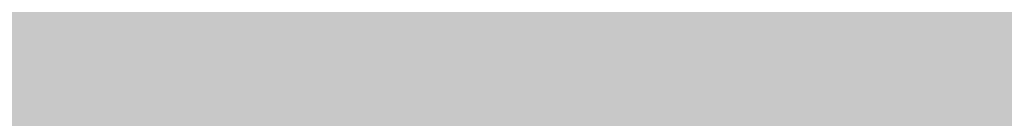
# Model space of a CAD drawing. Units: millimetres. Extents: x -22994 to 29398, y -19990 to 20176.
# Tile 99 of 135: x 229.428 to 230.597, y 84.615 to 84.732. Entities that reach past the tile are written whole.
import ezdxf
from ezdxf import colors
from ezdxf.entities.mleader import LeaderData, LeaderLine
from ezdxf.math import Vec2, Vec3

# ---------------------------------------------------------------- set-up
doc = ezdxf.new("R2010")
doc.units = ezdxf.units.MM
doc.header["$MEASUREMENT"] = 0
doc.layers.add('M-ANNO-TEXT', color=7, linetype='Continuous', lineweight=25)
doc.layers.add('M-DIMS', color=2, linetype='Continuous', lineweight=18)
doc.styles.get("Standard").update_dxf_attribs({"font": 'arial.ttf'})
doc.dimstyles.get("Standard").update_dxf_attribs({"dimtxt": 0.18, "dimasz": 10000, "dimexe": 0.18, "dimexo": 0.0625, "dimgap": 0.09, "dimtad": 0, "dimtih": 1, "dimtoh": 1, "dimdec": 0, "dimzin": 0, "dimdsep": 46, "dimtxsty": 'Standard', "dimcen": 0.09, "dimadec": 0, "dimazin": 0, "dimtfac": 1, "dimtdec": 0, "dimtofl": 0, "dimtmove": 0, "dimatfit": 3, "dimfxl": 1, "dimtolj": 1, "dimtzin": 0, "dimlwd": 30, "dimarcsym": 0})

# ---------------------------------------------------------------- blocks, each defined once
blk = doc.blocks.new('*D2')
at = {"layer": 'Defpoints', "color": 0, "transparency": 16777216}
for p in [(6.6773, 10.2713), (290.852, 10.2713), (290.852, -5.0787)]:
    blk.add_point(p, dxfattribs=at)
at = {"layer": 'M-DIMS', "color": 0, "lineweight": -2, "transparency": 16777216}
for p, q in [((6.6773, 10.2088), (6.6773, -5.2587)), ((290.852, 10.2088), (290.852, -5.2587))]:
    blk.add_line(p, q, dxfattribs=at)
at = {"layer": 'M-DIMS', "color": 0, "lineweight": 30, "transparency": 16777216}
for p, q in [((-9993.3227, -5.0787), (-19993.3227, -5.0787)), ((10290.852, -5.0787), (20290.852, -5.0787))]:
    blk.add_line(p, q, dxfattribs=at)
at = {"layer": 'M-DIMS', "color": 0, "transparency": 16777216}
for points in [[(-9993.3227, 1661.5879), (-9993.3227, -1671.7454), (6.6773, -5.0787)], [(10290.852, 1661.5879), (10290.852, -1671.7454), (290.852, -5.0787)]]:
    blk.add_solid(points, dxfattribs=at)
at = {"layer": 'M-DIMS', "color": 0, "transparency": 16777216, "insert": (148.7647, -5.0787), "char_height": 0.18, "attachment_point": 5}
blk.add_mtext('\\A1;284.2', dxfattribs=at)
blk = doc.blocks.new('*D3')
at = {"layer": 'Defpoints', "color": 0, "transparency": 16777216}
for p in [(110.2647, 204.1654), (110.2647, 176.3662), (95.8327, 127.967)]:
    blk.add_point(p, dxfattribs=at)
at = {"layer": 'M-DIMS', "color": 0, "lineweight": -2, "transparency": 16777216}
for p, q in [((95.8327, 128.0295), (95.8327, 204.3454)), ((110.2647, 176.4287), (110.2647, 204.3454))]:
    blk.add_line(p, q, dxfattribs=at)
at = {"layer": 'M-DIMS', "color": 0, "lineweight": 30, "transparency": 16777216}
for p, q in [((-9904.1673, 204.1654), (-19904.1673, 204.1654)), ((10110.2647, 204.1654), (20110.2647, 204.1654))]:
    blk.add_line(p, q, dxfattribs=at)
at = {"layer": 'M-DIMS', "color": 0, "transparency": 16777216}
for points in [[(-9904.1673, 1870.8321), (-9904.1673, -1462.5013), (95.8327, 204.1654)], [(10110.2647, 1870.8321), (10110.2647, -1462.5013), (110.2647, 204.1654)]]:
    blk.add_solid(points, dxfattribs=at)
at = {"layer": 'M-DIMS', "color": 0, "transparency": 16777216, "insert": (103.0487, 204.1654), "char_height": 0.18, "attachment_point": 5}
blk.add_mtext('\\A1;14.432', dxfattribs=at)
blk = doc.blocks.new('*D4')
at = {"layer": 'Defpoints', "color": 0, "transparency": 16777216}
for p in [(116.2647, 204.1654), (110.2647, 176.3662), (116.2647, 176.3662)]:
    blk.add_point(p, dxfattribs=at)
at = {"layer": 'M-DIMS', "color": 0, "lineweight": -2, "transparency": 16777216}
for p, q in [((110.2647, 176.4287), (110.2647, 204.3454)), ((116.2647, 176.4287), (116.2647, 204.3454))]:
    blk.add_line(p, q, dxfattribs=at)
at = {"layer": 'M-DIMS', "color": 0, "lineweight": 30, "transparency": 16777216}
for p, q in [((-9889.7353, 204.1654), (-19889.7353, 204.1654)), ((10116.2647, 204.1654), (20116.2647, 204.1654))]:
    blk.add_line(p, q, dxfattribs=at)
at = {"layer": 'M-DIMS', "color": 0, "transparency": 16777216}
for points in [[(-9889.7353, 1870.8321), (-9889.7353, -1462.5013), (110.2647, 204.1654)], [(10116.2647, 1870.8321), (10116.2647, -1462.5013), (116.2647, 204.1654)]]:
    blk.add_solid(points, dxfattribs=at)
at = {"layer": 'M-DIMS', "color": 0, "transparency": 16777216, "insert": (113.2647, 204.1654), "char_height": 0.18, "attachment_point": 5}
blk.add_mtext('\\A1;6', dxfattribs=at)
blk = doc.blocks.new('*D5')
at = {"layer": 'Defpoints', "color": 0, "transparency": 16777216}
for p in [(181.2647, 204.1654), (116.2647, 176.3662), (181.2647, 176.3662)]:
    blk.add_point(p, dxfattribs=at)
at = {"layer": 'M-DIMS', "color": 0, "lineweight": -2, "transparency": 16777216}
for p, q in [((116.2647, 176.4287), (116.2647, 204.3454)), ((181.2647, 176.4287), (181.2647, 204.3454))]:
    blk.add_line(p, q, dxfattribs=at)
at = {"layer": 'M-DIMS', "color": 0, "lineweight": 30, "transparency": 16777216}
for p, q in [((-9883.7353, 204.1654), (-19883.7353, 204.1654)), ((10181.2647, 204.1654), (20181.2647, 204.1654))]:
    blk.add_line(p, q, dxfattribs=at)
at = {"layer": 'M-DIMS', "color": 0, "transparency": 16777216}
for points in [[(-9883.7353, 1870.8321), (-9883.7353, -1462.5013), (116.2647, 204.1654)], [(10181.2647, 1870.8321), (10181.2647, -1462.5013), (181.2647, 204.1654)]]:
    blk.add_solid(points, dxfattribs=at)
at = {"layer": 'M-DIMS', "color": 0, "transparency": 16777216, "insert": (148.7647, 204.1654), "char_height": 0.18, "attachment_point": 5}
blk.add_mtext('\\A1;65', dxfattribs=at)
blk = doc.blocks.new('*D6')
at = {"layer": 'Defpoints', "color": 0, "transparency": 16777216}
for p in [(187.2647, 204.1654), (181.2647, 176.3662), (187.2647, 176.3662)]:
    blk.add_point(p, dxfattribs=at)
at = {"layer": 'M-DIMS', "color": 0, "lineweight": -2, "transparency": 16777216}
for p, q in [((181.2647, 176.4287), (181.2647, 204.3454)), ((187.2647, 176.4287), (187.2647, 204.3454))]:
    blk.add_line(p, q, dxfattribs=at)
at = {"layer": 'M-DIMS', "color": 0, "lineweight": 30, "transparency": 16777216}
for p, q in [((-9818.7353, 204.1654), (-19818.7353, 204.1654)), ((10187.2647, 204.1654), (20187.2647, 204.1654))]:
    blk.add_line(p, q, dxfattribs=at)
at = {"layer": 'M-DIMS', "color": 0, "transparency": 16777216}
for points in [[(-9818.7353, 1870.8321), (-9818.7353, -1462.5013), (181.2647, 204.1654)], [(10187.2647, 1870.8321), (10187.2647, -1462.5013), (187.2647, 204.1654)]]:
    blk.add_solid(points, dxfattribs=at)
at = {"layer": 'M-DIMS', "color": 0, "transparency": 16777216, "insert": (184.2647, 204.1654), "char_height": 0.18, "attachment_point": 5}
blk.add_mtext('\\A1;6', dxfattribs=at)
blk = doc.blocks.new('*D7')
at = {"layer": 'Defpoints', "color": 0, "transparency": 16777216}
for p in [(201.6967, 204.1654), (187.2647, 176.3662), (201.6967, 127.967)]:
    blk.add_point(p, dxfattribs=at)
at = {"layer": 'M-DIMS', "color": 0, "lineweight": -2, "transparency": 16777216}
for p, q in [((187.2647, 176.4287), (187.2647, 204.3454)), ((201.6967, 128.0295), (201.6967, 204.3454))]:
    blk.add_line(p, q, dxfattribs=at)
at = {"layer": 'M-DIMS', "color": 0, "lineweight": 30, "transparency": 16777216}
for p, q in [((-9812.7353, 204.1654), (-19812.7353, 204.1654)), ((10201.6967, 204.1654), (20201.6967, 204.1654))]:
    blk.add_line(p, q, dxfattribs=at)
at = {"layer": 'M-DIMS', "color": 0, "transparency": 16777216}
for points in [[(-9812.7353, 1870.8321), (-9812.7353, -1462.5013), (187.2647, 204.1654)], [(10201.6967, 1870.8321), (10201.6967, -1462.5013), (201.6967, 204.1654)]]:
    blk.add_solid(points, dxfattribs=at)
at = {"layer": 'M-DIMS', "color": 0, "transparency": 16777216, "insert": (194.4807, 204.1654), "char_height": 0.18, "attachment_point": 5}
blk.add_mtext('\\A1;14.432', dxfattribs=at)
blk = doc.blocks.new('*D8')
at = {"layer": 'Defpoints', "color": 0, "transparency": 16777216}
for p in [(227.6485, 204.1654), (227.6485, 146.7296), (201.6967, 127.967)]:
    blk.add_point(p, dxfattribs=at)
at = {"layer": 'M-DIMS', "color": 0, "lineweight": -2, "transparency": 16777216}
for p, q in [((201.6967, 128.0295), (201.6967, 204.3454)), ((227.6485, 146.7921), (227.6485, 204.3454))]:
    blk.add_line(p, q, dxfattribs=at)
at = {"layer": 'M-DIMS', "color": 0, "lineweight": 30, "transparency": 16777216}
for p, q in [((-9798.3033, 204.1654), (-19798.3033, 204.1654)), ((10227.6485, 204.1654), (20227.6485, 204.1654))]:
    blk.add_line(p, q, dxfattribs=at)
at = {"layer": 'M-DIMS', "color": 0, "transparency": 16777216}
for points in [[(-9798.3033, 1870.8321), (-9798.3033, -1462.5013), (201.6967, 204.1654)], [(10227.6485, 1870.8321), (10227.6485, -1462.5013), (227.6485, 204.1654)]]:
    blk.add_solid(points, dxfattribs=at)
at = {"layer": 'M-DIMS', "color": 0, "transparency": 16777216, "insert": (214.6726, 204.1654), "char_height": 0.18, "attachment_point": 5}
blk.add_mtext('\\A1;25.95', dxfattribs=at)
blk = doc.blocks.new('*D9')
at = {"layer": 'Defpoints', "color": 0, "transparency": 16777216}
for p in [(187.2647, 176.3662), (306.202, 176.3662), (290.852, 10.2713)]:
    blk.add_point(p, dxfattribs=at)
at = {"layer": 'M-DIMS', "color": 0, "lineweight": 30, "transparency": 16777216}
for p, q in [((306.202, 10176.3662), (306.202, 20176.3662)), ((306.202, -9989.7287), (306.202, -19989.7287))]:
    blk.add_line(p, q, dxfattribs=at)
at = {"layer": 'M-DIMS', "color": 0, "lineweight": -2, "transparency": 16777216}
for p, q in [((187.3272, 176.3662), (306.382, 176.3662)), ((290.9145, 10.2713), (306.382, 10.2713))]:
    blk.add_line(p, q, dxfattribs=at)
at = {"layer": 'M-DIMS', "color": 0, "transparency": 16777216}
for points in [[(-1360.4646, 10176.3662), (1972.8687, 10176.3662), (306.202, 176.3662)], [(-1360.4646, -9989.7287), (1972.8687, -9989.7287), (306.202, 10.2713)]]:
    blk.add_solid(points, dxfattribs=at)
at = {"layer": 'M-DIMS', "color": 0, "transparency": 16777216, "insert": (306.202, 93.3187), "char_height": 0.18, "attachment_point": 5}
blk.add_mtext('\\A1;166.1', dxfattribs=at)
blk = doc.blocks.new('*D10')
at = {"layer": 'Defpoints', "color": 0, "transparency": 16777216}
for p in [(125.6498, 136.0713), (133.3459, 136.0713), (133.3459, -5.0787)]:
    blk.add_point(p, dxfattribs=at)
at = {"layer": 'M-DIMS', "color": 0, "lineweight": -2, "transparency": 16777216}
for p, q in [((125.6498, 136.0088), (125.6498, -5.2587)), ((133.3459, 136.0088), (133.3459, -5.2587))]:
    blk.add_line(p, q, dxfattribs=at)
at = {"layer": 'M-DIMS', "color": 0, "lineweight": 30, "transparency": 16777216}
for p, q in [((-9874.3502, -5.0787), (-19874.3502, -5.0787)), ((10133.3459, -5.0787), (20133.3459, -5.0787))]:
    blk.add_line(p, q, dxfattribs=at)
at = {"layer": 'M-DIMS', "color": 0, "transparency": 16777216}
for points in [[(-9874.3502, 1661.5879), (-9874.3502, -1671.7454), (125.6498, -5.0787)], [(10133.3459, 1661.5879), (10133.3459, -1671.7454), (133.3459, -5.0787)]]:
    blk.add_solid(points, dxfattribs=at)
at = {"layer": 'M-DIMS', "color": 0, "transparency": 16777216, "insert": (129.4978, -5.0787), "char_height": 0.18, "attachment_point": 5}
blk.add_mtext('\\A1;7.696', dxfattribs=at)
blk = doc.blocks.new('*D11')
at = {"layer": 'Defpoints', "color": 0, "transparency": 16777216}
for p in [(133.3459, 136.0713), (135.6498, 136.0713), (135.6498, -5.0787)]:
    blk.add_point(p, dxfattribs=at)
at = {"layer": 'M-DIMS', "color": 0, "lineweight": -2, "transparency": 16777216}
for p, q in [((133.3459, 136.0088), (133.3459, -5.2587)), ((135.6498, 136.0088), (135.6498, -5.2587))]:
    blk.add_line(p, q, dxfattribs=at)
at = {"layer": 'M-DIMS', "color": 0, "lineweight": 30, "transparency": 16777216}
for p, q in [((-9866.6541, -5.0787), (-19866.6541, -5.0787)), ((10135.6498, -5.0787), (20135.6498, -5.0787))]:
    blk.add_line(p, q, dxfattribs=at)
at = {"layer": 'M-DIMS', "color": 0, "transparency": 16777216}
for points in [[(-9866.6541, 1661.5879), (-9866.6541, -1671.7454), (133.3459, -5.0787)], [(10135.6498, 1661.5879), (10135.6498, -1671.7454), (135.6498, -5.0787)]]:
    blk.add_solid(points, dxfattribs=at)
at = {"layer": 'M-DIMS', "color": 0, "transparency": 16777216, "insert": (134.4978, -5.0787), "char_height": 0.18, "attachment_point": 5}
blk.add_mtext('\\A1;2.304', dxfattribs=at)
blk = doc.blocks.new('*D12')
at = {"layer": 'Defpoints', "color": 0, "transparency": 16777216}
for p in [(135.6498, 136.0713), (145.6498, 136.0713), (145.6498, -5.0787)]:
    blk.add_point(p, dxfattribs=at)
at = {"layer": 'M-DIMS', "color": 0, "lineweight": -2, "transparency": 16777216}
for p, q in [((135.6498, 136.0088), (135.6498, -5.2587)), ((145.6498, 136.0088), (145.6498, -5.2587))]:
    blk.add_line(p, q, dxfattribs=at)
at = {"layer": 'M-DIMS', "color": 0, "lineweight": 30, "transparency": 16777216}
for p, q in [((-9864.3502, -5.0787), (-19864.3502, -5.0787)), ((10145.6498, -5.0787), (20145.6498, -5.0787))]:
    blk.add_line(p, q, dxfattribs=at)
at = {"layer": 'M-DIMS', "color": 0, "transparency": 16777216}
for points in [[(-9864.3502, 1661.5879), (-9864.3502, -1671.7454), (135.6498, -5.0787)], [(10145.6498, 1661.5879), (10145.6498, -1671.7454), (145.6498, -5.0787)]]:
    blk.add_solid(points, dxfattribs=at)
at = {"layer": 'M-DIMS', "color": 0, "transparency": 16777216, "insert": (140.6498, -5.0787), "char_height": 0.18, "attachment_point": 5}
blk.add_mtext('\\A1;10', dxfattribs=at)
blk = doc.blocks.new('*D13')
at = {"layer": 'Defpoints', "color": 0, "transparency": 16777216}
for p in [(145.6498, 136.0713), (155.6498, 136.0713), (155.6498, -5.0787)]:
    blk.add_point(p, dxfattribs=at)
at = {"layer": 'M-DIMS', "color": 0, "lineweight": -2, "transparency": 16777216}
for p, q in [((145.6498, 136.0088), (145.6498, -5.2587)), ((155.6498, 136.0088), (155.6498, -5.2587))]:
    blk.add_line(p, q, dxfattribs=at)
at = {"layer": 'M-DIMS', "color": 0, "lineweight": 30, "transparency": 16777216}
for p, q in [((-9854.3502, -5.0787), (-19854.3502, -5.0787)), ((10155.6498, -5.0787), (20155.6498, -5.0787))]:
    blk.add_line(p, q, dxfattribs=at)
at = {"layer": 'M-DIMS', "color": 0, "transparency": 16777216}
for points in [[(-9854.3502, 1661.5879), (-9854.3502, -1671.7454), (145.6498, -5.0787)], [(10155.6498, 1661.5879), (10155.6498, -1671.7454), (155.6498, -5.0787)]]:
    blk.add_solid(points, dxfattribs=at)
at = {"layer": 'M-DIMS', "color": 0, "transparency": 16777216, "insert": (150.6498, -5.0787), "char_height": 0.18, "attachment_point": 5}
blk.add_mtext('\\A1;10', dxfattribs=at)
blk = doc.blocks.new('*D14')
at = {"layer": 'Defpoints', "color": 0, "transparency": 16777216}
for p in [(155.6498, 136.0713), (165.6498, 136.0713), (165.6498, -5.0787)]:
    blk.add_point(p, dxfattribs=at)
at = {"layer": 'M-DIMS', "color": 0, "lineweight": -2, "transparency": 16777216}
for p, q in [((155.6498, 136.0088), (155.6498, -5.2587)), ((165.6498, 136.0088), (165.6498, -5.2587))]:
    blk.add_line(p, q, dxfattribs=at)
at = {"layer": 'M-DIMS', "color": 0, "lineweight": 30, "transparency": 16777216}
for p, q in [((-9844.3502, -5.0787), (-19844.3502, -5.0787)), ((10165.6498, -5.0787), (20165.6498, -5.0787))]:
    blk.add_line(p, q, dxfattribs=at)
at = {"layer": 'M-DIMS', "color": 0, "transparency": 16777216}
for points in [[(-9844.3502, 1661.5879), (-9844.3502, -1671.7454), (155.6498, -5.0787)], [(10165.6498, 1661.5879), (10165.6498, -1671.7454), (165.6498, -5.0787)]]:
    blk.add_solid(points, dxfattribs=at)
at = {"layer": 'M-DIMS', "color": 0, "transparency": 16777216, "insert": (160.6498, -5.0787), "char_height": 0.18, "attachment_point": 5}
blk.add_mtext('\\A1;10', dxfattribs=at)
blk = doc.blocks.new('*D15')
at = {"layer": 'Defpoints', "color": 0, "transparency": 16777216}
for p in [(173.3459, 154.788), (173.3459, 136.0713), (306.202, 136.0713)]:
    blk.add_point(p, dxfattribs=at)
at = {"layer": 'M-DIMS', "color": 0, "lineweight": 30, "transparency": 16777216}
for p, q in [((306.202, 10154.788), (306.202, 20154.788)), ((306.202, -9863.9287), (306.202, -19863.9287))]:
    blk.add_line(p, q, dxfattribs=at)
at = {"layer": 'M-DIMS', "color": 0, "lineweight": -2, "transparency": 16777216}
for p, q in [((173.4084, 154.788), (306.382, 154.788)), ((173.4084, 136.0713), (306.382, 136.0713))]:
    blk.add_line(p, q, dxfattribs=at)
at = {"layer": 'M-DIMS', "color": 0, "transparency": 16777216}
for points in [[(-1360.4646, 10154.788), (1972.8687, 10154.788), (306.202, 154.788)], [(-1360.4646, -9863.9287), (1972.8687, -9863.9287), (306.202, 136.0713)]]:
    blk.add_solid(points, dxfattribs=at)
at = {"layer": 'M-DIMS', "color": 0, "transparency": 16777216, "insert": (306.202, 145.4297), "char_height": 0.18, "attachment_point": 5}
blk.add_mtext('\\A1;18.717', dxfattribs=at)
blk = doc.blocks.new('*D16')
at = {"layer": 'Defpoints', "color": 0, "transparency": 16777216}
for p in [(120.1702, 204.1654), (110.4658, 48.0349), (120.1702, 48.0349)]:
    blk.add_point(p, dxfattribs=at)
at = {"layer": 'M-DIMS', "color": 0, "lineweight": -2, "transparency": 16777216}
for p, q in [((110.4658, 48.0974), (110.4658, 204.3454)), ((120.1702, 48.0974), (120.1702, 204.3454))]:
    blk.add_line(p, q, dxfattribs=at)
at = {"layer": 'M-DIMS', "color": 0, "lineweight": 30, "transparency": 16777216}
for p, q in [((-9889.5342, 204.1654), (-19889.5342, 204.1654)), ((10120.1702, 204.1654), (20120.1702, 204.1654))]:
    blk.add_line(p, q, dxfattribs=at)
at = {"layer": 'M-DIMS', "color": 0, "transparency": 16777216}
for points in [[(-9889.5342, 1870.8321), (-9889.5342, -1462.5013), (110.4658, 204.1654)], [(10120.1702, 1870.8321), (10120.1702, -1462.5013), (120.1702, 204.1654)]]:
    blk.add_solid(points, dxfattribs=at)
at = {"layer": 'M-DIMS', "color": 0, "transparency": 16777216, "insert": (115.318, 204.1654), "char_height": 0.18, "attachment_point": 5}
blk.add_mtext('\\A1;9.704', dxfattribs=at)
blk = doc.blocks.new('*D17')
at = {"layer": 'Defpoints', "color": 0, "transparency": 16777216}
for p in [(126.1702, 204.1654), (120.1702, 48.0349), (126.1702, 48.0349)]:
    blk.add_point(p, dxfattribs=at)
at = {"layer": 'M-DIMS', "color": 0, "lineweight": -2, "transparency": 16777216}
for p, q in [((120.1702, 48.0974), (120.1702, 204.3454)), ((126.1702, 48.0974), (126.1702, 204.3454))]:
    blk.add_line(p, q, dxfattribs=at)
at = {"layer": 'M-DIMS', "color": 0, "lineweight": 30, "transparency": 16777216}
for p, q in [((-9879.8298, 204.1654), (-19879.8298, 204.1654)), ((10126.1702, 204.1654), (20126.1702, 204.1654))]:
    blk.add_line(p, q, dxfattribs=at)
at = {"layer": 'M-DIMS', "color": 0, "transparency": 16777216}
for points in [[(-9879.8298, 1870.8321), (-9879.8298, -1462.5013), (120.1702, 204.1654)], [(10126.1702, 1870.8321), (10126.1702, -1462.5013), (126.1702, 204.1654)]]:
    blk.add_solid(points, dxfattribs=at)
at = {"layer": 'M-DIMS', "color": 0, "transparency": 16777216, "insert": (123.1702, 204.1654), "char_height": 0.18, "attachment_point": 5}
blk.add_mtext('\\A1;6', dxfattribs=at)
blk = doc.blocks.new('*D18')
at = {"layer": 'Defpoints', "color": 0, "transparency": 16777216}
for p in [(132.1702, 204.1654), (126.1702, 48.0349), (132.1702, 48.0349)]:
    blk.add_point(p, dxfattribs=at)
at = {"layer": 'M-DIMS', "color": 0, "lineweight": -2, "transparency": 16777216}
for p, q in [((126.1702, 48.0974), (126.1702, 204.3454)), ((132.1702, 48.0974), (132.1702, 204.3454))]:
    blk.add_line(p, q, dxfattribs=at)
at = {"layer": 'M-DIMS', "color": 0, "lineweight": 30, "transparency": 16777216}
for p, q in [((-9873.8298, 204.1654), (-19873.8298, 204.1654)), ((10132.1702, 204.1654), (20132.1702, 204.1654))]:
    blk.add_line(p, q, dxfattribs=at)
at = {"layer": 'M-DIMS', "color": 0, "transparency": 16777216}
for points in [[(-9873.8298, 1870.8321), (-9873.8298, -1462.5013), (126.1702, 204.1654)], [(10132.1702, 1870.8321), (10132.1702, -1462.5013), (132.1702, 204.1654)]]:
    blk.add_solid(points, dxfattribs=at)
at = {"layer": 'M-DIMS', "color": 0, "transparency": 16777216, "insert": (129.1702, 204.1654), "char_height": 0.18, "attachment_point": 5}
blk.add_mtext('\\A1;6', dxfattribs=at)
blk = doc.blocks.new('*D19')
at = {"layer": 'Defpoints', "color": 0, "transparency": 16777216}
for p in [(138.1702, 204.1654), (132.1702, 48.0349), (138.1702, 48.0349)]:
    blk.add_point(p, dxfattribs=at)
at = {"layer": 'M-DIMS', "color": 0, "lineweight": -2, "transparency": 16777216}
for p, q in [((132.1702, 48.0974), (132.1702, 204.3454)), ((138.1702, 48.0974), (138.1702, 204.3454))]:
    blk.add_line(p, q, dxfattribs=at)
at = {"layer": 'M-DIMS', "color": 0, "lineweight": 30, "transparency": 16777216}
for p, q in [((-9867.8298, 204.1654), (-19867.8298, 204.1654)), ((10138.1702, 204.1654), (20138.1702, 204.1654))]:
    blk.add_line(p, q, dxfattribs=at)
at = {"layer": 'M-DIMS', "color": 0, "transparency": 16777216}
for points in [[(-9867.8298, 1870.8321), (-9867.8298, -1462.5013), (132.1702, 204.1654)], [(10138.1702, 1870.8321), (10138.1702, -1462.5013), (138.1702, 204.1654)]]:
    blk.add_solid(points, dxfattribs=at)
at = {"layer": 'M-DIMS', "color": 0, "transparency": 16777216, "insert": (135.1702, 204.1654), "char_height": 0.18, "attachment_point": 5}
blk.add_mtext('\\A1;6', dxfattribs=at)
blk = doc.blocks.new('*D20')
at = {"layer": 'Defpoints', "color": 0, "transparency": 16777216}
for p in [(144.1702, 204.1654), (138.1702, 48.0349), (144.1702, 48.0349)]:
    blk.add_point(p, dxfattribs=at)
at = {"layer": 'M-DIMS', "color": 0, "lineweight": -2, "transparency": 16777216}
for p, q in [((138.1702, 48.0974), (138.1702, 204.3454)), ((144.1702, 48.0974), (144.1702, 204.3454))]:
    blk.add_line(p, q, dxfattribs=at)
at = {"layer": 'M-DIMS', "color": 0, "lineweight": 30, "transparency": 16777216}
for p, q in [((-9861.8298, 204.1654), (-19861.8298, 204.1654)), ((10144.1702, 204.1654), (20144.1702, 204.1654))]:
    blk.add_line(p, q, dxfattribs=at)
at = {"layer": 'M-DIMS', "color": 0, "transparency": 16777216}
for points in [[(-9861.8298, 1870.8321), (-9861.8298, -1462.5013), (138.1702, 204.1654)], [(10144.1702, 1870.8321), (10144.1702, -1462.5013), (144.1702, 204.1654)]]:
    blk.add_solid(points, dxfattribs=at)
at = {"layer": 'M-DIMS', "color": 0, "transparency": 16777216, "insert": (141.1702, 204.1654), "char_height": 0.18, "attachment_point": 5}
blk.add_mtext('\\A1;6', dxfattribs=at)
blk = doc.blocks.new('*D21')
at = {"layer": 'Defpoints', "color": 0, "transparency": 16777216}
for p in [(149.1157, 204.1654), (144.1702, 48.0349), (149.1157, 48.0349)]:
    blk.add_point(p, dxfattribs=at)
at = {"layer": 'M-DIMS', "color": 0, "lineweight": -2, "transparency": 16777216}
for p, q in [((144.1702, 48.0974), (144.1702, 204.3454)), ((149.1157, 48.0974), (149.1157, 204.3454))]:
    blk.add_line(p, q, dxfattribs=at)
at = {"layer": 'M-DIMS', "color": 0, "lineweight": 30, "transparency": 16777216}
for p, q in [((-9855.8298, 204.1654), (-19855.8298, 204.1654)), ((10149.1157, 204.1654), (20149.1157, 204.1654))]:
    blk.add_line(p, q, dxfattribs=at)
at = {"layer": 'M-DIMS', "color": 0, "transparency": 16777216}
for points in [[(-9855.8298, 1870.8321), (-9855.8298, -1462.5013), (144.1702, 204.1654)], [(10149.1157, 1870.8321), (10149.1157, -1462.5013), (149.1157, 204.1654)]]:
    blk.add_solid(points, dxfattribs=at)
at = {"layer": 'M-DIMS', "color": 0, "transparency": 16777216, "insert": (146.6429, 204.1654), "char_height": 0.18, "attachment_point": 5}
blk.add_mtext('\\A1;4.945', dxfattribs=at)
blk = doc.blocks.new('*D22')
at = {"layer": 'Defpoints', "color": 0, "transparency": 16777216}
for p in [(149.1157, 30.9895), (155.1157, 30.9895), (155.1157, -5.0787)]:
    blk.add_point(p, dxfattribs=at)
at = {"layer": 'M-DIMS', "color": 0, "lineweight": -2, "transparency": 16777216}
for p, q in [((149.1157, 30.927), (149.1157, -5.2587)), ((155.1157, 30.927), (155.1157, -5.2587))]:
    blk.add_line(p, q, dxfattribs=at)
at = {"layer": 'M-DIMS', "color": 0, "lineweight": 30, "transparency": 16777216}
for p, q in [((-9850.8843, -5.0787), (-19850.8843, -5.0787)), ((10155.1157, -5.0787), (20155.1157, -5.0787))]:
    blk.add_line(p, q, dxfattribs=at)
at = {"layer": 'M-DIMS', "color": 0, "transparency": 16777216}
for points in [[(-9850.8843, 1661.5879), (-9850.8843, -1671.7454), (149.1157, -5.0787)], [(10155.1157, 1661.5879), (10155.1157, -1671.7454), (155.1157, -5.0787)]]:
    blk.add_solid(points, dxfattribs=at)
at = {"layer": 'M-DIMS', "color": 0, "transparency": 16777216, "insert": (152.1157, -5.0787), "char_height": 0.18, "attachment_point": 5}
blk.add_mtext('\\A1;6', dxfattribs=at)
blk = doc.blocks.new('*D23')
at = {"layer": 'Defpoints', "color": 0, "transparency": 16777216}
for p in [(155.1157, 30.9895), (161.1157, 30.9895), (161.1157, -5.0787)]:
    blk.add_point(p, dxfattribs=at)
at = {"layer": 'M-DIMS', "color": 0, "lineweight": -2, "transparency": 16777216}
for p, q in [((155.1157, 30.927), (155.1157, -5.2587)), ((161.1157, 30.927), (161.1157, -5.2587))]:
    blk.add_line(p, q, dxfattribs=at)
at = {"layer": 'M-DIMS', "color": 0, "lineweight": 30, "transparency": 16777216}
for p, q in [((-9844.8843, -5.0787), (-19844.8843, -5.0787)), ((10161.1157, -5.0787), (20161.1157, -5.0787))]:
    blk.add_line(p, q, dxfattribs=at)
at = {"layer": 'M-DIMS', "color": 0, "transparency": 16777216}
for points in [[(-9844.8843, 1661.5879), (-9844.8843, -1671.7454), (155.1157, -5.0787)], [(10161.1157, 1661.5879), (10161.1157, -1671.7454), (161.1157, -5.0787)]]:
    blk.add_solid(points, dxfattribs=at)
at = {"layer": 'M-DIMS', "color": 0, "transparency": 16777216, "insert": (158.1157, -5.0787), "char_height": 0.18, "attachment_point": 5}
blk.add_mtext('\\A1;6', dxfattribs=at)
blk = doc.blocks.new('*D24')
at = {"layer": 'Defpoints', "color": 0, "transparency": 16777216}
for p in [(161.1157, 30.9895), (166.4387, 30.9895), (166.4387, -5.0787)]:
    blk.add_point(p, dxfattribs=at)
at = {"layer": 'M-DIMS', "color": 0, "lineweight": -2, "transparency": 16777216}
for p, q in [((161.1157, 30.927), (161.1157, -5.2587)), ((166.4387, 30.927), (166.4387, -5.2587))]:
    blk.add_line(p, q, dxfattribs=at)
at = {"layer": 'M-DIMS', "color": 0, "lineweight": 30, "transparency": 16777216}
for p, q in [((-9838.8843, -5.0787), (-19838.8843, -5.0787)), ((10166.4387, -5.0787), (20166.4387, -5.0787))]:
    blk.add_line(p, q, dxfattribs=at)
at = {"layer": 'M-DIMS', "color": 0, "transparency": 16777216}
for points in [[(-9838.8843, 1661.5879), (-9838.8843, -1671.7454), (161.1157, -5.0787)], [(10166.4387, 1661.5879), (10166.4387, -1671.7454), (166.4387, -5.0787)]]:
    blk.add_solid(points, dxfattribs=at)
at = {"layer": 'M-DIMS', "color": 0, "transparency": 16777216, "insert": (163.7772, -5.0787), "char_height": 0.18, "attachment_point": 5}
blk.add_mtext('\\A1;5.323', dxfattribs=at)
blk = doc.blocks.new('*D25')
at = {"layer": 'Defpoints', "color": 0, "transparency": 16777216}
for p in [(166.4387, 30.9895), (172.4387, 30.9895), (172.4387, -5.0787)]:
    blk.add_point(p, dxfattribs=at)
at = {"layer": 'M-DIMS', "color": 0, "lineweight": -2, "transparency": 16777216}
for p, q in [((166.4387, 30.927), (166.4387, -5.2587)), ((172.4387, 30.927), (172.4387, -5.2587))]:
    blk.add_line(p, q, dxfattribs=at)
at = {"layer": 'M-DIMS', "color": 0, "lineweight": 30, "transparency": 16777216}
for p, q in [((-9833.5613, -5.0787), (-19833.5613, -5.0787)), ((10172.4387, -5.0787), (20172.4387, -5.0787))]:
    blk.add_line(p, q, dxfattribs=at)
at = {"layer": 'M-DIMS', "color": 0, "transparency": 16777216}
for points in [[(-9833.5613, 1661.5879), (-9833.5613, -1671.7454), (166.4387, -5.0787)], [(10172.4387, 1661.5879), (10172.4387, -1671.7454), (172.4387, -5.0787)]]:
    blk.add_solid(points, dxfattribs=at)
at = {"layer": 'M-DIMS', "color": 0, "transparency": 16777216, "insert": (169.4387, -5.0787), "char_height": 0.18, "attachment_point": 5}
blk.add_mtext('\\A1;6', dxfattribs=at)
blk = doc.blocks.new('*D26')
at = {"layer": 'Defpoints', "color": 0, "transparency": 16777216}
for p in [(172.4387, 30.9895), (178.4387, 30.9895), (178.4387, -5.0787)]:
    blk.add_point(p, dxfattribs=at)
at = {"layer": 'M-DIMS', "color": 0, "lineweight": -2, "transparency": 16777216}
for p, q in [((172.4387, 30.927), (172.4387, -5.2587)), ((178.4387, 30.927), (178.4387, -5.2587))]:
    blk.add_line(p, q, dxfattribs=at)
at = {"layer": 'M-DIMS', "color": 0, "lineweight": 30, "transparency": 16777216}
for p, q in [((-9827.5613, -5.0787), (-19827.5613, -5.0787)), ((10178.4387, -5.0787), (20178.4387, -5.0787))]:
    blk.add_line(p, q, dxfattribs=at)
at = {"layer": 'M-DIMS', "color": 0, "transparency": 16777216}
for points in [[(-9827.5613, 1661.5879), (-9827.5613, -1671.7454), (172.4387, -5.0787)], [(10178.4387, 1661.5879), (10178.4387, -1671.7454), (178.4387, -5.0787)]]:
    blk.add_solid(points, dxfattribs=at)
at = {"layer": 'M-DIMS', "color": 0, "transparency": 16777216, "insert": (175.4387, -5.0787), "char_height": 0.18, "attachment_point": 5}
blk.add_mtext('\\A1;6', dxfattribs=at)
blk = doc.blocks.new('*D27')
at = {"layer": 'Defpoints', "color": 0, "transparency": 16777216}
for p in [(178.4387, 30.9895), (188.1175, 30.9895), (188.1175, -5.0787)]:
    blk.add_point(p, dxfattribs=at)
at = {"layer": 'M-DIMS', "color": 0, "lineweight": -2, "transparency": 16777216}
for p, q in [((178.4387, 30.927), (178.4387, -5.2587)), ((188.1175, 30.927), (188.1175, -5.2587))]:
    blk.add_line(p, q, dxfattribs=at)
at = {"layer": 'M-DIMS', "color": 0, "lineweight": 30, "transparency": 16777216}
for p, q in [((-9821.5613, -5.0787), (-19821.5613, -5.0787)), ((10188.1175, -5.0787), (20188.1175, -5.0787))]:
    blk.add_line(p, q, dxfattribs=at)
at = {"layer": 'M-DIMS', "color": 0, "transparency": 16777216}
for points in [[(-9821.5613, 1661.5879), (-9821.5613, -1671.7454), (178.4387, -5.0787)], [(10188.1175, 1661.5879), (10188.1175, -1671.7454), (188.1175, -5.0787)]]:
    blk.add_solid(points, dxfattribs=at)
at = {"layer": 'M-DIMS', "color": 0, "transparency": 16777216, "insert": (183.2781, -5.0787), "char_height": 0.18, "attachment_point": 5}
blk.add_mtext('\\A1;9.679', dxfattribs=at)
blk = doc.blocks.new('*D28')
at = {"layer": 'Defpoints', "color": 0, "transparency": 16777216}
for p in [(188.1175, 48.0349), (306.202, 48.0349), (188.1175, 30.9895)]:
    blk.add_point(p, dxfattribs=at)
at = {"layer": 'M-DIMS', "color": 0, "lineweight": 30, "transparency": 16777216}
for p, q in [((306.202, 10048.0349), (306.202, 20048.0349)), ((306.202, -9969.0105), (306.202, -19969.0105))]:
    blk.add_line(p, q, dxfattribs=at)
at = {"layer": 'M-DIMS', "color": 0, "lineweight": -2, "transparency": 16777216}
for p, q in [((188.18, 48.0349), (306.382, 48.0349)), ((188.18, 30.9895), (306.382, 30.9895))]:
    blk.add_line(p, q, dxfattribs=at)
at = {"layer": 'M-DIMS', "color": 0, "transparency": 16777216}
for points in [[(-1360.4646, 10048.0349), (1972.8687, 10048.0349), (306.202, 48.0349)], [(-1360.4646, -9969.0105), (1972.8687, -9969.0105), (306.202, 30.9895)]]:
    blk.add_solid(points, dxfattribs=at)
at = {"layer": 'M-DIMS', "color": 0, "transparency": 16777216, "insert": (306.202, 39.5122), "char_height": 0.18, "attachment_point": 5}
blk.add_mtext('\\A1;17.045', dxfattribs=at)
blk = doc.blocks.new('*D29')
at = {"layer": 'Defpoints', "color": 0, "transparency": 16777216}
for p in [(36.8006, 80.045), (64.0296, 80.045)]:
    blk.add_point(p, dxfattribs=at)
at = {"layer": 'M-DIMS', "color": 0, "lineweight": -2, "transparency": 16777216}
for p, q in [((50.4151, 79.955), (50.4151, 80.135)), ((50.3251, 80.045), (50.5051, 80.045))]:
    blk.add_line(p, q, dxfattribs=at)
at = {"layer": 'M-DIMS', "color": 0, "lineweight": 30, "transparency": 16777216}
blk.add_line((20064.0296, 80.0303), (10064.0296, 80.0377), dxfattribs=at)
at = {"layer": 'M-DIMS', "color": 0, "transparency": 16777216}
blk.add_solid([(10064.0309, 1746.7043), (10064.0284, -1586.629), (64.0296, 80.045)], dxfattribs=at)
at = {"layer": 'M-DIMS', "color": 0, "transparency": 16777216, "insert": (20064.5213, 80.0303), "char_height": 0.18, "attachment_point": 5}
blk.add_mtext('\\A1;∅27.23', dxfattribs=at)
blk = doc.blocks.new('*D30')
at = {"layer": 'Defpoints', "color": 0, "transparency": 16777216}
for p in [(216.3148, 146.7291), (238.9821, 146.73)]:
    blk.add_point(p, dxfattribs=at)
at = {"layer": 'M-DIMS', "color": 0, "lineweight": 30, "transparency": 16777216}
blk.add_line((20238.9821, 147.4959), (10238.9821, 147.1129), dxfattribs=at)
at = {"layer": 'M-DIMS', "color": 0, "lineweight": -2, "transparency": 16777216}
for p, q in [((227.6485, 146.6396), (227.6485, 146.8196)), ((227.5585, 146.7296), (227.7385, 146.7296))]:
    blk.add_line(p, q, dxfattribs=at)
at = {"layer": 'M-DIMS', "color": 0, "transparency": 16777216}
blk.add_solid([(10238.9183, 1813.7796), (10239.0459, -1519.5537), (238.9821, 146.73)], dxfattribs=at)
at = {"layer": 'M-DIMS', "color": 0, "transparency": 16777216, "insert": (20239.5436, 147.4959), "char_height": 0.18, "attachment_point": 5}
blk.add_mtext('\\A1;∅22.667', dxfattribs=at)
blk = doc.blocks.new('*D31')
at = {"layer": 'Defpoints', "color": 0, "transparency": 16777216}
for p in [(223.1641, 146.7291), (232.1328, 146.73)]:
    blk.add_point(p, dxfattribs=at)
at = {"layer": 'M-DIMS', "color": 0, "lineweight": 30, "transparency": 16777216}
blk.add_line((20232.1327, 148.6656), (10232.1328, 147.6978), dxfattribs=at)
at = {"layer": 'M-DIMS', "color": 0, "lineweight": -2, "transparency": 16777216}
for p, q in [((227.6485, 146.6396), (227.6485, 146.8196)), ((227.5585, 146.7296), (227.7385, 146.7296))]:
    blk.add_line(p, q, dxfattribs=at)
at = {"layer": 'M-DIMS', "color": 0, "transparency": 16777216}
blk.add_solid([(10231.9715, 1814.3645), (10232.2941, -1518.9688), (232.1328, 146.73)], dxfattribs=at)
at = {"layer": 'M-DIMS', "color": 0, "transparency": 16777216, "insert": (20232.6245, 148.6656), "char_height": 0.18, "attachment_point": 5}
blk.add_mtext('\\A1;∅8.969', dxfattribs=at)
blk = doc.blocks.new('*D33')
at = {"layer": 'Defpoints', "color": 0, "transparency": 16777216}
for p in [(229.5613, 154.3773), (232.9972, 153.3509)]:
    blk.add_point(p, dxfattribs=at)
at = {"layer": 'M-DIMS', "color": 0, "lineweight": -2, "transparency": 16777216}
for p, q in [((229.5613, 154.2873), (229.5613, 154.4673)), ((229.4713, 154.3773), (229.6513, 154.3773))]:
    blk.add_line(p, q, dxfattribs=at)
at = {"layer": 'M-DIMS', "color": 0, "lineweight": 30, "transparency": 16777216}
for p, q in [((19396.3388, -5570.8378), (9814.668, -2708.7434)), ((29396.3388, -5570.8378), (19396.3388, -5570.8378))]:
    blk.add_line(p, q, dxfattribs=at)
at = {"layer": 'M-DIMS', "color": 0, "transparency": 16777216}
blk.add_solid([(10291.6837, -1111.7983), (9337.6523, -4305.6886), (232.9972, 153.3509)], dxfattribs=at)
at = {"layer": 'M-DIMS', "color": 0, "transparency": 16777216, "insert": (29397.0125, -5570.8378), "char_height": 0.18, "attachment_point": 5}
blk.add_mtext('\\A1;6X R3.586', dxfattribs=at)
blk = doc.blocks.new('*D36')
at = {"layer": 'Defpoints', "color": 0, "transparency": 16777216}
for p in [(46.39, 31.3035), (46.3875, 26.5934)]:
    blk.add_point(p, dxfattribs=at)
at = {"layer": 'M-DIMS', "color": 0, "lineweight": 30, "transparency": 16777216}
for p, q in [((57.1499, 20031.3006), (51.77, 10031.302)), ((10057.1499, 20031.3006), (57.1499, 20031.3006))]:
    blk.add_line(p, q, dxfattribs=at)
at = {"layer": 'M-DIMS', "color": 0, "lineweight": -2, "transparency": 16777216}
for p, q in [((46.3887, 28.8585), (46.3887, 29.0385)), ((46.2987, 28.9485), (46.4787, 28.9485))]:
    blk.add_line(p, q, dxfattribs=at)
at = {"layer": 'M-DIMS', "color": 0, "transparency": 16777216}
blk.add_solid([(-1614.8965, 10032.1987), (1718.4364, 10030.4054), (46.39, 31.3035)], dxfattribs=at)
at = {"layer": 'M-DIMS', "color": 0, "transparency": 16777216, "insert": (10057.5542, 20031.3006), "char_height": 0.18, "attachment_point": 5}
blk.add_mtext('\\A1;∅4.71', dxfattribs=at)
blk = doc.blocks.new('*D37')
at = {"layer": 'Defpoints', "color": 0, "transparency": 16777216}
for p in [(54.8343, 118.6145), (59.4936, 118.614)]:
    blk.add_point(p, dxfattribs=at)
at = {"layer": 'M-DIMS', "color": 0, "lineweight": -2, "transparency": 16777216}
for p, q in [((57.1639, 118.5243), (57.1639, 118.7043)), ((57.0739, 118.6143), (57.2539, 118.6143))]:
    blk.add_line(p, q, dxfattribs=at)
at = {"layer": 'M-DIMS', "color": 0, "lineweight": 30, "transparency": 16777216}
blk.add_line((20059.4934, 116.2531), (10059.4935, 117.4336), dxfattribs=at)
at = {"layer": 'M-DIMS', "color": 0, "transparency": 16777216}
blk.add_solid([(10059.6902, 1784.1002), (10059.2968, -1549.2331), (59.4936, 118.614)], dxfattribs=at)
at = {"layer": 'M-DIMS', "color": 0, "transparency": 16777216, "insert": (20059.9852, 116.2531), "char_height": 0.18, "attachment_point": 5}
blk.add_mtext('\\A1;∅4.659', dxfattribs=at)

msp = doc.modelspace()

# ---------------------------------------------------------------- dimensions: what is measured, and where the dimension line sits
at = {"layer": 'M-DIMS'}
for base, p1, p2, override, picture, middle in [((306.202, 176.3662), (290.852, 10.2713), (187.2647, 176.3662), {"dimdec": 1, "dimlfac": 1, "dimrnd": 0, "dimzin": 0, "dimdsep": 46, "dimlunit": 2}, '*D9', (306.202, 93.3187)), ((306.202, 136.0713), (173.3459, 154.788), (173.3459, 136.0713), {"dimdec": 3, "dimlfac": 1, "dimrnd": 0, "dimzin": 0, "dimdsep": 46, "dimlunit": 2}, '*D15', (306.202, 145.4297)), ((306.202, 48.0349), (188.1175, 30.9895), (188.1175, 48.0349), {"dimdec": 3, "dimlfac": 1, "dimrnd": 0, "dimzin": 0, "dimdsep": 46, "dimlunit": 2}, '*D28', (306.202, 39.5122))]:
    dim = msp.add_linear_dim(base=base, p1=p1, p2=p2, angle=90, dimstyle='Standard', override=override, dxfattribs=at)
    dim.commit()
    dim.dimension.update_dxf_attribs({"geometry": picture, "text_midpoint": middle})
for p1, p2, override, picture, middle in [((46.3875, 26.5934), (46.39, 31.3035), {"dimdec": 2, "dimlfac": 1, "dimrnd": 0, "dimzin": 0, "dimdsep": 46, "dimlunit": 2}, '*D36', (10057.5542, 20031.3006)), ((223.1641, 146.7291), (232.1328, 146.73), {"dimdec": 3, "dimlfac": 1, "dimrnd": 0, "dimzin": 0, "dimdsep": 46, "dimlunit": 2}, '*D31', (20232.1327, 148.6656)), ((216.3148, 146.7291), (238.9821, 146.73), {"dimdec": 3, "dimlfac": 1, "dimrnd": 0, "dimzin": 0, "dimdsep": 46, "dimlunit": 2}, '*D30', (20238.9821, 147.4959))]:
    dim = msp.add_diameter_dim_2p(p1=p1, p2=p2, dimstyle='Standard', override=override, dxfattribs=at)
    dim.commit()
    dim.dimension.update_dxf_attribs({"geometry": picture, "text_midpoint": middle, "dimtype": 163})
for base, p1, p2, override, picture, middle in [((110.2647, 204.1654), (95.8327, 127.967), (110.2647, 176.3662), {"dimdec": 3, "dimlfac": 1, "dimrnd": 0, "dimzin": 0, "dimdsep": 46, "dimlunit": 2}, '*D3', (103.0487, 204.1654)), ((116.2647, 204.1654), (110.2647, 176.3662), (116.2647, 176.3662), {"dimdec": 0, "dimlfac": 1, "dimrnd": 0, "dimzin": 0, "dimdsep": 46, "dimlunit": 2}, '*D4', (113.2647, 204.1654)), ((120.1702, 204.1654), (110.4658, 48.0349), (120.1702, 48.0349), {"dimdec": 3, "dimlfac": 1, "dimrnd": 0, "dimzin": 0, "dimdsep": 46, "dimlunit": 2}, '*D16', (115.318, 204.1654)), ((181.2647, 204.1654), (116.2647, 176.3662), (181.2647, 176.3662), {"dimdec": 0, "dimlfac": 1, "dimrnd": 0, "dimzin": 0, "dimdsep": 46, "dimlunit": 2}, '*D5', (148.7647, 204.1654)), ((126.1702, 204.1654), (120.1702, 48.0349), (126.1702, 48.0349), {"dimdec": 0, "dimlfac": 1, "dimrnd": 0, "dimzin": 0, "dimdsep": 46, "dimlunit": 2}, '*D17', (123.1702, 204.1654)), ((132.1702, 204.1654), (126.1702, 48.0349), (132.1702, 48.0349), {"dimdec": 0, "dimlfac": 1, "dimrnd": 0, "dimzin": 0, "dimdsep": 46, "dimlunit": 2}, '*D18', (129.1702, 204.1654)), ((138.1702, 204.1654), (132.1702, 48.0349), (138.1702, 48.0349), {"dimdec": 0, "dimlfac": 1, "dimrnd": 0, "dimzin": 0, "dimdsep": 46, "dimlunit": 2}, '*D19', (135.1702, 204.1654)), ((144.1702, 204.1654), (138.1702, 48.0349), (144.1702, 48.0349), {"dimdec": 0, "dimlfac": 1, "dimrnd": 0, "dimzin": 0, "dimdsep": 46, "dimlunit": 2}, '*D20', (141.1702, 204.1654)), ((149.11567, 204.16539), (144.17023, 48.03494), (149.11567, 48.03494), {"dimdec": 3, "dimlfac": 1, "dimrnd": 0, "dimzin": 0, "dimdsep": 46, "dimlunit": 2}, '*D21', (146.64295, 204.16539)), ((187.2647, 204.1654), (181.2647, 176.3662), (187.2647, 176.3662), {"dimdec": 0, "dimlfac": 1, "dimrnd": 0, "dimzin": 0, "dimdsep": 46, "dimlunit": 2}, '*D6', (184.2647, 204.1654)), ((201.6967, 204.1654), (187.2647, 176.3662), (201.6967, 127.967), {"dimdec": 3, "dimlfac": 1, "dimrnd": 0, "dimzin": 0, "dimdsep": 46, "dimlunit": 2}, '*D7', (194.4807, 204.1654)), ((227.6485, 204.1654), (201.6967, 127.967), (227.6485, 146.7296), {"dimdec": 2, "dimlfac": 1, "dimrnd": 0, "dimzin": 0, "dimdsep": 46, "dimlunit": 2}, '*D8', (214.6726, 204.1654)), ((290.852, -5.0787), (6.6773, 10.2713), (290.852, 10.2713), {"dimdec": 1, "dimlfac": 1, "dimrnd": 0, "dimzin": 0, "dimdsep": 46, "dimlunit": 2}, '*D2', (148.7647, -5.0787)), ((133.3459, -5.0787), (125.6498, 136.0713), (133.3459, 136.0713), {"dimdec": 3, "dimlfac": 1, "dimrnd": 0, "dimzin": 0, "dimdsep": 46, "dimlunit": 2}, '*D10', (129.4978, -5.0787)), ((135.6498, -5.0787), (133.3459, 136.0713), (135.6498, 136.0713), {"dimdec": 3, "dimlfac": 1, "dimrnd": 0, "dimzin": 0, "dimdsep": 46, "dimlunit": 2}, '*D11', (134.4978, -5.0787)), ((145.6498, -5.0787), (135.6498, 136.0713), (145.6498, 136.0713), {"dimdec": 0, "dimlfac": 1, "dimrnd": 0, "dimzin": 0, "dimdsep": 46, "dimlunit": 2}, '*D12', (140.6498, -5.0787)), ((155.6498, -5.0787), (145.6498, 136.0713), (155.6498, 136.0713), {"dimdec": 0, "dimlfac": 1, "dimrnd": 0, "dimzin": 0, "dimdsep": 46, "dimlunit": 2}, '*D13', (150.6498, -5.0787)), ((155.1157, -5.0787), (149.1157, 30.9895), (155.1157, 30.9895), {"dimdec": 0, "dimlfac": 1, "dimrnd": 0, "dimzin": 0, "dimdsep": 46, "dimlunit": 2}, '*D22', (152.1157, -5.0787)), ((161.1157, -5.0787), (155.1157, 30.9895), (161.1157, 30.9895), {"dimdec": 0, "dimlfac": 1, "dimrnd": 0, "dimzin": 0, "dimdsep": 46, "dimlunit": 2}, '*D23', (158.1157, -5.0787)), ((165.6498, -5.0787), (155.6498, 136.0713), (165.6498, 136.0713), {"dimdec": 0, "dimlfac": 1, "dimrnd": 0, "dimzin": 0, "dimdsep": 46, "dimlunit": 2}, '*D14', (160.6498, -5.0787)), ((166.4387, -5.0787), (161.1157, 30.9895), (166.4387, 30.9895), {"dimdec": 3, "dimlfac": 1, "dimrnd": 0, "dimzin": 0, "dimdsep": 46, "dimlunit": 2}, '*D24', (163.7772, -5.0787)), ((172.4387, -5.0787), (166.4387, 30.9895), (172.4387, 30.9895), {"dimdec": 0, "dimlfac": 1, "dimrnd": 0, "dimzin": 0, "dimdsep": 46, "dimlunit": 2}, '*D25', (169.4387, -5.0787)), ((178.4387, -5.0787), (172.4387, 30.9895), (178.4387, 30.9895), {"dimdec": 0, "dimlfac": 1, "dimrnd": 0, "dimzin": 0, "dimdsep": 46, "dimlunit": 2}, '*D26', (175.4387, -5.0787)), ((188.1175, -5.0787), (178.4387, 30.9895), (188.1175, 30.9895), {"dimdec": 3, "dimlfac": 1, "dimrnd": 0, "dimzin": 0, "dimdsep": 46, "dimlunit": 2}, '*D27', (183.2781, -5.0787))]:
    dim = msp.add_linear_dim(base=base, p1=p1, p2=p2, dimstyle='Standard', override=override, dxfattribs=at)
    dim.commit()
    dim.dimension.update_dxf_attribs({"geometry": picture, "text_midpoint": middle})
for p1, p2, override, picture, middle in [((54.8343, 118.6145), (59.4936, 118.614), {"dimdec": 3, "dimlfac": 1, "dimrnd": 0, "dimzin": 0, "dimdsep": 46, "dimlunit": 2}, '*D37', (20059.4934, 116.2531)), ((36.8006, 80.045), (64.0296, 80.045), {"dimdec": 2, "dimlfac": 1, "dimrnd": 0, "dimzin": 0, "dimdsep": 46, "dimlunit": 2}, '*D29', (20064.0296, 80.0303))]:
    dim = msp.add_diameter_dim_2p(p1=p1, p2=p2, dimstyle='Standard', override=override, dxfattribs=at)
    dim.commit()
    dim.dimension.update_dxf_attribs({"geometry": picture, "text_midpoint": middle})
dim = msp.add_radius_dim(center=(229.5613, 154.3773), mpoint=(232.9972, 153.3509), text='6X <>', dimstyle='Standard', override={"dimdec": 3, "dimlfac": 1, "dimrnd": 0, "dimzin": 0, "dimdsep": 46, "dimlunit": 2}, dxfattribs=at)
dim.commit()
dim.dimension.update_dxf_attribs({"geometry": '*D33', "text_midpoint": (29397.0125, -5570.8378)})

# ---------------------------------------------------------------- leaders
at = {"layer": 'M-ANNO-TEXT'}
ml = msp.add_multileader_mtext('Standard', dxfattribs=at)
ml.set_content('combustion chamber', color=256)
ml.set_leader_properties()
ml.build(insert=Vec2(0, 0))
ml.multileader.update_dxf_attribs({"dogleg_length": 0.36, "arrow_head_size": 200})
ctx = ml.context
ctx.base_point, ctx.char_height, ctx.arrow_head_size, ctx.landing_gap_size, ctx.plane_origin = Vec3(215.7321, 57.9149), 3, 200, 0.09, Vec3(189.1175, 57.9149)
notes = []
notes.append((ctx, [(0, (1, 1, 0), (215.3721, 57.9149), (1, 0), 0.36, [(0, [(189.1175, 57.9149)], 0, [])])]))
ctx.mtext.insert, ctx.mtext.flow_direction = Vec3(215.8221, 59.4394), 5
for ctx, leaders in notes:
    for number, flags, end, landing, length, lines in leaders:
        leader = LeaderData()
        leader.index, (leader.has_last_leader_line, leader.has_dogleg_vector, leader.attachment_direction) = number, flags
        leader.last_leader_point, leader.dogleg_vector, leader.dogleg_length = Vec3(end), Vec3(landing), length
        for number, points, colour, breaks in lines:
            line = LeaderLine()
            line.index, line.vertices, line.color, line.breaks = number, Vec3.list(points), colors.encode_raw_color(colour), breaks
            leader.lines.append(line)
        ctx.leaders.append(leader)

doc.saveas('drawing.dxf')
